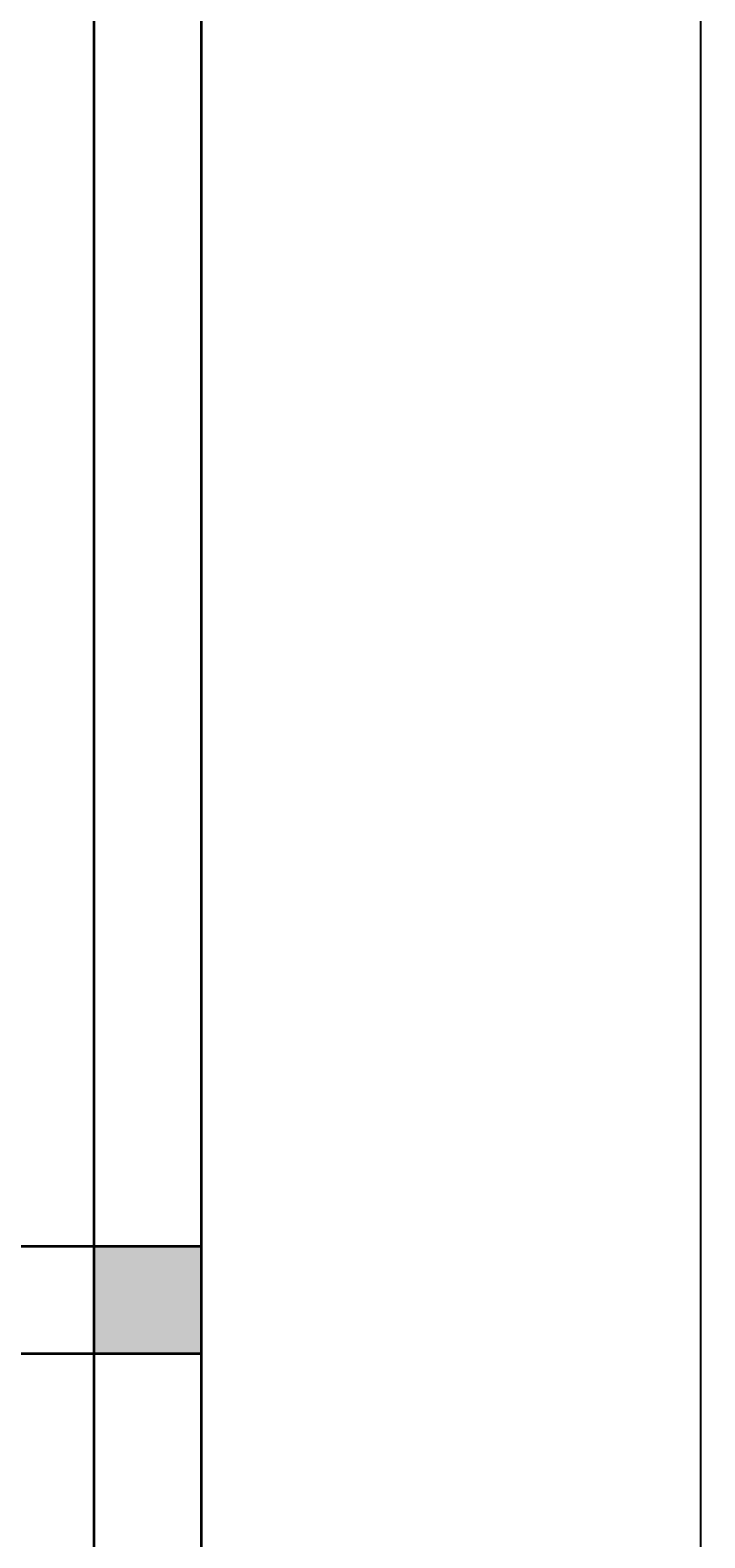
# Model space of a CAD drawing. Units: inches. Extents: x -36302355 to 648, y -221479757 to 75.
# Tile 21 of 37: x 591 to 647, y -595 to -469. Entities that reach past the tile are written whole.
import ezdxf

# ---------------------------------------------------------------- set-up
doc = ezdxf.new("R2010")
doc.units = ezdxf.units.IN
doc.header["$MEASUREMENT"] = 0
for name, color, linetype, lineweight in [('A-ANNO-DIMS', 2, 'Continuous', 18), ('A-COLS-PATT', 242, 'Continuous', 13), ('A-WALL', 7, 'Continuous', 35)]:
    doc.layers.add(name, color=color, linetype=linetype, lineweight=lineweight)
doc.styles.get("Standard").update_dxf_attribs({"font": 'arial.ttf'})
doc.dimstyles.get("Standard").update_dxf_attribs({"dimtxt": 0.18, "dimasz": 0.18, "dimexe": 0.18, "dimexo": 0.0625, "dimgap": 0.09, "dimtad": 0, "dimtih": 1, "dimtoh": 1, "dimdec": 0, "dimzin": 0, "dimdsep": 46, "dimlunit": 3, "dimtxsty": 'Standard', "dimcen": 0.09, "dimadec": 0, "dimazin": 0, "dimtfac": 1, "dimtdec": 0, "dimtofl": 0, "dimtmove": 0, "dimatfit": 3, "dimfxl": 1, "dimtolj": 1, "dimtzin": 0, "dimarcsym": 0})

# ---------------------------------------------------------------- blocks, each defined once
blk = doc.blocks.new('*D57')
at = {"layer": 'A-ANNO-DIMS', "color": 0, "lineweight": -2, "transparency": 16777216}
for p, q in [((605.26, 24.98), (647.33, 24.98)), ((647.15, 24.8), (647.15, -348.34)), ((647.15, -721.84), (647.15, -348.7)), ((605.26, -722.02), (647.33, -722.02))]:
    blk.add_line(p, q, dxfattribs=at)
at = {"layer": 'A-ANNO-DIMS', "color": 0, "transparency": 16777216}
for points in [[(647.12, 24.8), (647.18, 24.8), (647.15, 24.98)], [(647.12, -721.84), (647.18, -721.84), (647.15, -722.02)]]:
    blk.add_solid(points, dxfattribs=at)
at = {"layer": 'Defpoints', "color": 0, "transparency": 16777216}
for p in [(605.2, 24.98), (605.2, -722.02), (647.15, -722.02)]:
    blk.add_point(p, dxfattribs=at)
at = {"layer": 'A-ANNO-DIMS', "color": 0, "transparency": 16777216, "insert": (647.15, -348.52), "char_height": 0.18, "attachment_point": 5}
blk.add_mtext('\\A1;62\'-3"', dxfattribs=at)

msp = doc.modelspace()

# ---------------------------------------------------------------- hatches: boundary and pattern name
at = {"layer": 'A-COLS-PATT'}
h = msp.add_hatch(color=256, dxfattribs=at)
h.dxf.hatch_style = 1
h.paths.add_polyline_path([(605.2, -571.02), (596.2, -571.02), (596.2, -580.02), (605.2, -580.02)])
h.paths.add_polyline_path([(605.2, -374.52), (596.2, -374.52), (596.2, -379.02), (605.2, -379.02)])

# ---------------------------------------------------------------- linework, layer by layer
at = {"layer": 'A-WALL'}
for p, q in [((605.2, 24.98), (605.2, -722.02)), ((596.2, -431.02), (596.2, -722.02)), ((335.2, -571.02), (605.2, -571.02)), ((335.2, -580.02), (605.2, -580.02))]:
    msp.add_line(p, q, dxfattribs=at)

# ---------------------------------------------------------------- dimensions: what is measured, and where the dimension line sits
at = {"layer": 'A-ANNO-DIMS'}
dim = msp.add_linear_dim(base=(647.15, -722.02), p1=(605.2, 24.98), p2=(605.2, -722.02), angle=90, dimstyle='Standard', override={"dimdec": 1, "dimlfac": 1, "dimrnd": 0, "dimzin": 1, "dimdsep": 46, "dimlunit": 4, "dimfrac": 2}, dxfattribs=at)
dim.commit()
dim.dimension.update_dxf_attribs({"geometry": '*D57', "text_midpoint": (647.15, -348.52)})

doc.saveas('drawing.dxf')
